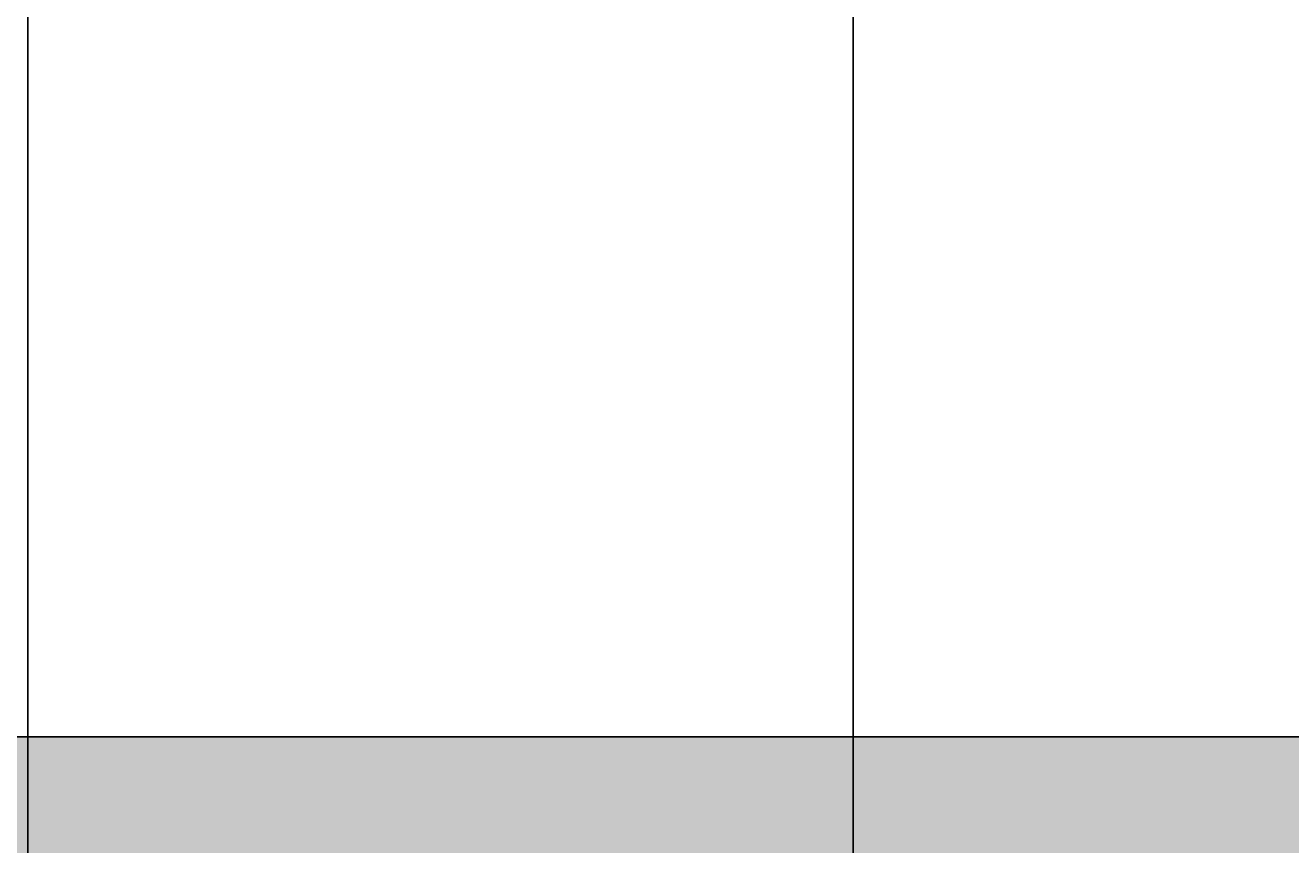
# Model space of a CAD drawing. Units: millimetres. Extents: x -11 to 280, y -4 to 208.
# Tile 44 of 55: x 151 to 186, y 106 to 128. Entities that reach past the tile are written whole.
import ezdxf

# ---------------------------------------------------------------- set-up
doc = ezdxf.new("R2010")
doc.units = ezdxf.units.MM
doc.layers.add('M-DIMS', color=2, linetype='Continuous', lineweight=18)
doc.layers.add('M-HYDR-PRES', color=7, linetype='Continuous', lineweight=25)
doc.layers.add('M-HYDR-PRES-PATT', color=240, linetype='Continuous', lineweight=13, true_color=0xed1f24)
doc.styles.get("Standard").update_dxf_attribs({"font": 'arial.ttf'})
doc.dimstyles.get("Standard").update_dxf_attribs({"dimtxt": 0.18, "dimasz": 0.18, "dimexe": 0.18, "dimexo": 0.0625, "dimgap": 0.09, "dimtad": 0, "dimtih": 1, "dimtoh": 1, "dimdec": 4, "dimzin": 0, "dimdsep": 46, "dimtxsty": 'Standard', "dimcen": 0.09, "dimadec": 0, "dimazin": 0, "dimtfac": 1, "dimtdec": 4, "dimtofl": 0, "dimtmove": 0, "dimatfit": 3, "dimfxl": 1, "dimtolj": 1, "dimtzin": 0, "dimarcsym": 0})

# ---------------------------------------------------------------- blocks, each defined once
blk = doc.blocks.new('*D5')
at = {"layer": 'Defpoints', "color": 0, "transparency": 16777216}
for p in [(24.759, 192.645), (-10.087, 11.435), (261.686, 11.435)]:
    blk.add_point(p, dxfattribs=at)
at = {"layer": 'M-DIMS', "color": 0, "lineweight": -2, "transparency": 16777216}
for p, q in [((24.696, 192.645), (-10.267, 192.645)), ((-10.087, 192.465), (-10.087, 102.222)), ((-10.087, 11.615), (-10.087, 101.858)), ((261.624, 11.435), (-10.267, 11.435))]:
    blk.add_line(p, q, dxfattribs=at)
at = {"layer": 'M-DIMS', "color": 0, "transparency": 16777216}
for points in [[(-10.117, 192.465), (-10.057, 192.465), (-10.087, 192.645)], [(-10.117, 11.615), (-10.057, 11.615), (-10.087, 11.435)]]:
    blk.add_solid(points, dxfattribs=at)
at = {"layer": 'M-DIMS', "color": 0, "transparency": 16777216, "insert": (-10.087, 102.04), "char_height": 0.18, "attachment_point": 5}
blk.add_mtext('\\A1;181.2', dxfattribs=at)
blk = doc.blocks.new('*D12')
at = {"layer": 'Defpoints', "color": 0, "transparency": 16777216}
for p in [(173.804, 207.495), (118.514, 96.485), (173.804, 89.387)]:
    blk.add_point(p, dxfattribs=at)
at = {"layer": 'M-DIMS', "color": 0, "lineweight": -2, "transparency": 16777216}
for p, q in [((118.514, 96.547), (118.514, 207.675)), ((118.694, 207.495), (145.765, 207.495)), ((173.624, 207.495), (146.553, 207.495)), ((173.804, 89.45), (173.804, 207.675))]:
    blk.add_line(p, q, dxfattribs=at)
at = {"layer": 'M-DIMS', "color": 0, "transparency": 16777216}
for points in [[(118.694, 207.525), (118.694, 207.465), (118.514, 207.495)], [(173.624, 207.525), (173.624, 207.465), (173.804, 207.495)]]:
    blk.add_solid(points, dxfattribs=at)
at = {"layer": 'M-DIMS', "color": 0, "transparency": 16777216, "insert": (146.159, 207.495), "char_height": 0.18, "attachment_point": 5}
blk.add_mtext('\\A1;55.29', dxfattribs=at)
blk = doc.blocks.new('*D18')
at = {"layer": 'Defpoints', "color": 0, "transparency": 16777216}
for p in [(173.804, 207.495), (173.804, 65.064), (151.022, 43.599)]:
    blk.add_point(p, dxfattribs=at)
at = {"layer": 'M-DIMS', "color": 0, "lineweight": -2, "transparency": 16777216}
for p, q in [((151.022, 43.662), (151.022, 207.675)), ((151.202, 207.495), (162.017, 207.495)), ((173.624, 207.495), (162.808, 207.495)), ((173.804, 65.126), (173.804, 207.675))]:
    blk.add_line(p, q, dxfattribs=at)
at = {"layer": 'M-DIMS', "color": 0, "transparency": 16777216}
for points in [[(151.202, 207.525), (151.202, 207.465), (151.022, 207.495)], [(173.624, 207.525), (173.624, 207.465), (173.804, 207.495)]]:
    blk.add_solid(points, dxfattribs=at)
at = {"layer": 'M-DIMS', "color": 0, "transparency": 16777216, "insert": (162.413, 207.495), "char_height": 0.18, "attachment_point": 5}
blk.add_mtext('\\A1;22.78', dxfattribs=at)
blk = doc.blocks.new('*D20')
at = {"layer": 'Defpoints', "color": 0, "transparency": 16777216}
for p in [(231.68, 207.495), (151.022, 43.599), (231.68, 43.599)]:
    blk.add_point(p, dxfattribs=at)
at = {"layer": 'M-DIMS', "color": 0, "lineweight": -2, "transparency": 16777216}
for p, q in [((151.022, 43.662), (151.022, 207.675)), ((151.202, 207.495), (190.957, 207.495)), ((231.5, 207.495), (191.745, 207.495)), ((231.68, 43.662), (231.68, 207.675))]:
    blk.add_line(p, q, dxfattribs=at)
at = {"layer": 'M-DIMS', "color": 0, "transparency": 16777216}
for points in [[(151.202, 207.525), (151.202, 207.465), (151.022, 207.495)], [(231.5, 207.525), (231.5, 207.465), (231.68, 207.495)]]:
    blk.add_solid(points, dxfattribs=at)
at = {"layer": 'M-DIMS', "color": 0, "transparency": 16777216, "insert": (191.351, 207.495), "char_height": 0.18, "attachment_point": 5}
blk.add_mtext('\\A1;80.66', dxfattribs=at)

msp = doc.modelspace()

# ---------------------------------------------------------------- hatches: boundary and pattern name
at = {"layer": 'M-HYDR-PRES-PATT'}
h = msp.add_hatch(color=256, dxfattribs=at)
h.set_gradient(color1=(237, 31, 36), color2=(237, 31, 36), tint=1)
h.paths.add_polyline_path([(232.2, 133.1228), (228.7, 133.1228), (228.7, 108.8141), (102.7646, 108.8141), (102.7646, 105.3141), (232.2, 105.3141)])
h.paths.add_polyline_path([(128.8433, 105.3141), (125.3433, 105.3141), (125.3433, 91.7099, 1), (128.8433, 91.7099)])
h.paths.add_polyline_path([(229.1617, 78.7098), (196.7745, 78.7098, -0.4142136), (191.7745, 83.7098), (191.7745, 105.3141), (188.2745, 105.3141), (188.2745, 80.2098, 0.4142136), (193.2745, 75.2098), (225.6617, 75.2098), (225.6617, 43.5991), (229.1617, 43.5991)])
h.paths.add_polyline_path([(102.7646, 110.3704), (95.5776, 110.3704), (95.5776, 103.9022), (102.7646, 103.9022)])
h.paths.add_polyline_path([(100.7059, 107.2502), (99.1711, 106.3641), (99.1711, 106.8641), (97.1711, 106.8641), (97.1711, 107.6363), (99.1711, 107.6363), (99.1711, 108.1363)], flags=16)
h.paths.add_polyline_path([(234.6119, 138.4081), (226.5106, 138.4081), (226.5106, 133.1228), (234.6119, 133.1228)])
h.paths.add_polyline_path([(231.1963, 135.7055), (230.2965, 134.1786), (229.4241, 135.7213), (229.9241, 135.7168), (229.9418, 137.7167), (230.7141, 137.7099), (230.6963, 135.71)], flags=16)

# ---------------------------------------------------------------- linework, layer by layer
at = {"layer": 'M-HYDR-PRES'}
msp.add_lwpolyline([(228.7, 133.1228), (228.7, 108.8141), (102.7646, 108.8141)], dxfattribs=at)

# ---------------------------------------------------------------- dimensions: what is measured, and where the dimension line sits
at = {"layer": 'M-DIMS'}
for base, p1, p2, picture, middle in [((173.8038, 207.495), (118.5137, 96.4849), (173.8038, 89.3873), '*D12', (146.1587, 207.495)), ((173.8038, 207.495), (151.0217, 43.5991), (173.8038, 65.0638), '*D18', (162.4127, 207.495)), ((231.6803, 207.495), (151.0217, 43.5991), (231.6803, 43.5991), '*D20', (191.351, 207.495))]:
    dim = msp.add_linear_dim(base=base, p1=p1, p2=p2, dimstyle='Standard', override={"dimdec": 2, "dimlfac": 1, "dimrnd": 0, "dimzin": 0, "dimdsep": 46, "dimlunit": 2}, dxfattribs=at)
    dim.commit()
    dim.dimension.update_dxf_attribs({"geometry": picture, "text_midpoint": middle})
dim = msp.add_linear_dim(base=(-10.0865, 11.4346), p1=(24.7588, 192.645), p2=(261.6863, 11.4346), angle=90, dimstyle='Standard', override={"dimdec": 1, "dimlfac": 1, "dimrnd": 0, "dimzin": 0, "dimdsep": 46, "dimlunit": 2}, dxfattribs=at)
dim.commit()
dim.dimension.update_dxf_attribs({"geometry": '*D5', "text_midpoint": (-10.0865, 102.0398)})

doc.saveas('drawing.dxf')
